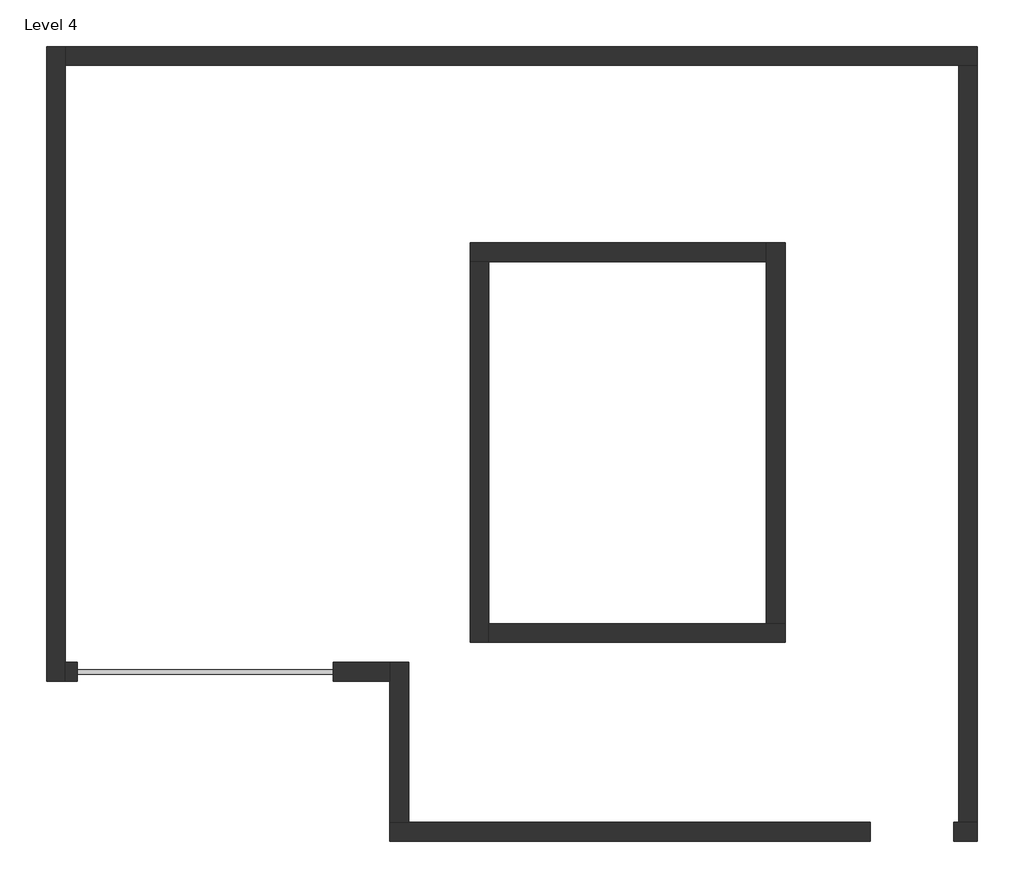
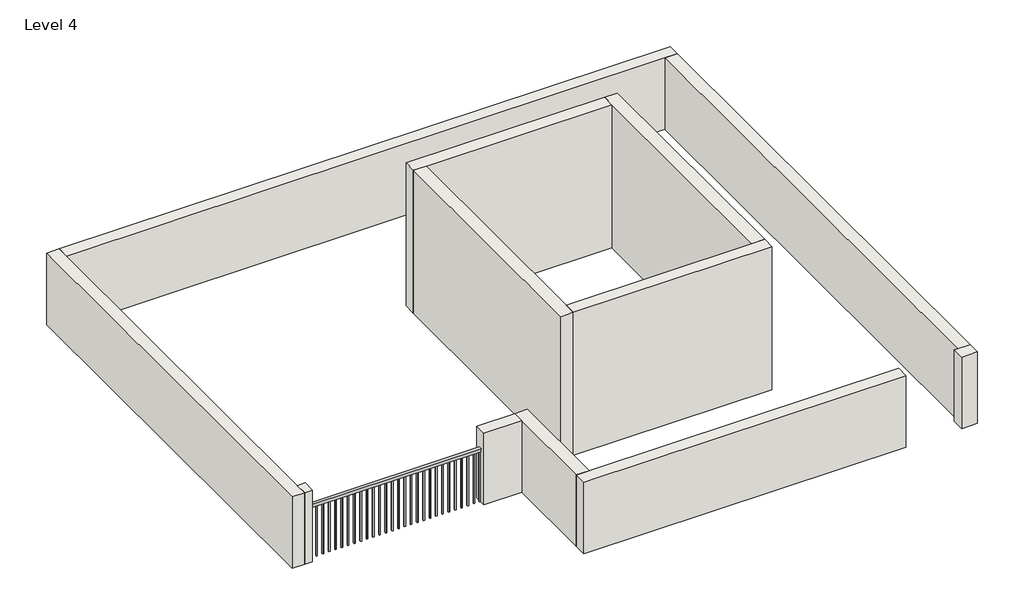
# One storey: 10 walls, 1 railing.
"""IFC4 building model written with IfcOpenShell, lengths in millimetres."""

from ifc_helpers import new_model, si_unit, frame, origin, place, context, project, spatial, polyline, outline, extrude, faceted_brep, element, save

model = new_model("IFC4")

# Units and contexts
model_context = context("Model", 3, world=origin())
ifc_project = project(units=[si_unit("LENGTHUNIT", "METRE", prefix="MILLI")], contexts=[model_context])

# Site, building, storey
site = spatial("IfcSite", under=ifc_project)
building = spatial("IfcBuilding", under=site)
storey = spatial("IfcBuildingStorey", under=building, Name="Level 4", Elevation=3810.0)

# Railing
placement = place(None, origin())
element("IfcRailing", 1, ObjectType="Handrail - Rectangular", at=placement, inside=storey, context=model_context, shape_type="SweptSolid", body=[
    extrude(outline(polyline([(-5551.2524032, 7396.0433441), (-5551.2524032, 7345.2433441), (-8317.8992801, 7345.2433441), (-8317.8992801, 7396.0433441), (-5551.2524032, 7396.0433441)])), frame((0.0, 0.0, 4673.6), z_axis=(0.0, 0.0, 1.0), x_axis=(1.0, 0.0, 0.0)), (0.0, 0.0, 1.0), 50.8),
    extrude(outline(polyline([(-8284.9274032, 7380.1683441), (-8284.9274032, 7361.1183441), (-8303.9774032, 7361.1183441), (-8303.9774032, 7380.1683441), (-8284.9274032, 7380.1683441)])), frame((0.0, 0.0, 3810.0), z_axis=(0.0, 0.0, 1.0), x_axis=(1.0, 0.0, 0.0)), (0.0, 0.0, 1.0), 863.6),
    extrude(outline(polyline([(-8183.3274032, 7380.1683441), (-8183.3274032, 7361.1183441), (-8202.3774032, 7361.1183441), (-8202.3774032, 7380.1683441), (-8183.3274032, 7380.1683441)])), frame((0.0, 0.0, 3810.0), z_axis=(0.0, 0.0, 1.0), x_axis=(1.0, 0.0, 0.0)), (0.0, 0.0, 1.0), 863.6),
    extrude(outline(polyline([(-8081.7274032, 7380.1683441), (-8081.7274032, 7361.1183441), (-8100.7774032, 7361.1183441), (-8100.7774032, 7380.1683441), (-8081.7274032, 7380.1683441)])), frame((0.0, 0.0, 3810.0), z_axis=(0.0, 0.0, 1.0), x_axis=(1.0, 0.0, 0.0)), (0.0, 0.0, 1.0), 863.6),
    extrude(outline(polyline([(-7980.1274032, 7380.1683441), (-7980.1274032, 7361.1183441), (-7999.1774032, 7361.1183441), (-7999.1774032, 7380.1683441), (-7980.1274032, 7380.1683441)])), frame((0.0, 0.0, 3810.0), z_axis=(0.0, 0.0, 1.0), x_axis=(1.0, 0.0, 0.0)), (0.0, 0.0, 1.0), 863.6),
    extrude(outline(polyline([(-7878.5274032, 7380.1683441), (-7878.5274032, 7361.1183441), (-7897.5774032, 7361.1183441), (-7897.5774032, 7380.1683441), (-7878.5274032, 7380.1683441)])), frame((0.0, 0.0, 3810.0), z_axis=(0.0, 0.0, 1.0), x_axis=(1.0, 0.0, 0.0)), (0.0, 0.0, 1.0), 863.6),
    extrude(outline(polyline([(-7776.9274032, 7380.1683441), (-7776.9274032, 7361.1183441), (-7795.9774032, 7361.1183441), (-7795.9774032, 7380.1683441), (-7776.9274032, 7380.1683441)])), frame((0.0, 0.0, 3810.0), z_axis=(0.0, 0.0, 1.0), x_axis=(1.0, 0.0, 0.0)), (0.0, 0.0, 1.0), 863.6),
    extrude(outline(polyline([(-7675.3274032, 7380.1683441), (-7675.3274032, 7361.1183441), (-7694.3774032, 7361.1183441), (-7694.3774032, 7380.1683441), (-7675.3274032, 7380.1683441)])), frame((0.0, 0.0, 3810.0), z_axis=(0.0, 0.0, 1.0), x_axis=(1.0, 0.0, 0.0)), (0.0, 0.0, 1.0), 863.6),
    extrude(outline(polyline([(-7573.7274032, 7380.1683441), (-7573.7274032, 7361.1183441), (-7592.7774032, 7361.1183441), (-7592.7774032, 7380.1683441), (-7573.7274032, 7380.1683441)])), frame((0.0, 0.0, 3810.0), z_axis=(0.0, 0.0, 1.0), x_axis=(1.0, 0.0, 0.0)), (0.0, 0.0, 1.0), 863.6),
    extrude(outline(polyline([(-7472.1274032, 7380.1683441), (-7472.1274032, 7361.1183441), (-7491.1774032, 7361.1183441), (-7491.1774032, 7380.1683441), (-7472.1274032, 7380.1683441)])), frame((0.0, 0.0, 3810.0), z_axis=(0.0, 0.0, 1.0), x_axis=(1.0, 0.0, 0.0)), (0.0, 0.0, 1.0), 863.6),
    extrude(outline(polyline([(-7370.5274032, 7380.1683441), (-7370.5274032, 7361.1183441), (-7389.5774032, 7361.1183441), (-7389.5774032, 7380.1683441), (-7370.5274032, 7380.1683441)])), frame((0.0, 0.0, 3810.0), z_axis=(0.0, 0.0, 1.0), x_axis=(1.0, 0.0, 0.0)), (0.0, 0.0, 1.0), 863.6),
    extrude(outline(polyline([(-7268.9274032, 7380.1683441), (-7268.9274032, 7361.1183441), (-7287.9774032, 7361.1183441), (-7287.9774032, 7380.1683441), (-7268.9274032, 7380.1683441)])), frame((0.0, 0.0, 3810.0), z_axis=(0.0, 0.0, 1.0), x_axis=(1.0, 0.0, 0.0)), (0.0, 0.0, 1.0), 863.6),
    extrude(outline(polyline([(-7167.3274032, 7380.1683441), (-7167.3274032, 7361.1183441), (-7186.3774032, 7361.1183441), (-7186.3774032, 7380.1683441), (-7167.3274032, 7380.1683441)])), frame((0.0, 0.0, 3810.0), z_axis=(0.0, 0.0, 1.0), x_axis=(1.0, 0.0, 0.0)), (0.0, 0.0, 1.0), 863.6),
    extrude(outline(polyline([(-7065.7274032, 7380.1683441), (-7065.7274032, 7361.1183441), (-7084.7774032, 7361.1183441), (-7084.7774032, 7380.1683441), (-7065.7274032, 7380.1683441)])), frame((0.0, 0.0, 3810.0), z_axis=(0.0, 0.0, 1.0), x_axis=(1.0, 0.0, 0.0)), (0.0, 0.0, 1.0), 863.6),
    extrude(outline(polyline([(-6964.1274032, 7380.1683441), (-6964.1274032, 7361.1183441), (-6983.1774032, 7361.1183441), (-6983.1774032, 7380.1683441), (-6964.1274032, 7380.1683441)])), frame((0.0, 0.0, 3810.0), z_axis=(0.0, 0.0, 1.0), x_axis=(1.0, 0.0, 0.0)), (0.0, 0.0, 1.0), 863.6),
    extrude(outline(polyline([(-6862.5274032, 7380.1683441), (-6862.5274032, 7361.1183441), (-6881.5774032, 7361.1183441), (-6881.5774032, 7380.1683441), (-6862.5274032, 7380.1683441)])), frame((0.0, 0.0, 3810.0), z_axis=(0.0, 0.0, 1.0), x_axis=(1.0, 0.0, 0.0)), (0.0, 0.0, 1.0), 863.6),
    extrude(outline(polyline([(-6760.9274032, 7380.1683441), (-6760.9274032, 7361.1183441), (-6779.9774032, 7361.1183441), (-6779.9774032, 7380.1683441), (-6760.9274032, 7380.1683441)])), frame((0.0, 0.0, 3810.0), z_axis=(0.0, 0.0, 1.0), x_axis=(1.0, 0.0, 0.0)), (0.0, 0.0, 1.0), 863.6),
    extrude(outline(polyline([(-6659.3274032, 7380.1683441), (-6659.3274032, 7361.1183441), (-6678.3774032, 7361.1183441), (-6678.3774032, 7380.1683441), (-6659.3274032, 7380.1683441)])), frame((0.0, 0.0, 3810.0), z_axis=(0.0, 0.0, 1.0), x_axis=(1.0, 0.0, 0.0)), (0.0, 0.0, 1.0), 863.6),
    extrude(outline(polyline([(-6557.7274032, 7380.1683441), (-6557.7274032, 7361.1183441), (-6576.7774032, 7361.1183441), (-6576.7774032, 7380.1683441), (-6557.7274032, 7380.1683441)])), frame((0.0, 0.0, 3810.0), z_axis=(0.0, 0.0, 1.0), x_axis=(1.0, 0.0, 0.0)), (0.0, 0.0, 1.0), 863.6),
    extrude(outline(polyline([(-6456.1274032, 7380.1683441), (-6456.1274032, 7361.1183441), (-6475.1774032, 7361.1183441), (-6475.1774032, 7380.1683441), (-6456.1274032, 7380.1683441)])), frame((0.0, 0.0, 3810.0), z_axis=(0.0, 0.0, 1.0), x_axis=(1.0, 0.0, 0.0)), (0.0, 0.0, 1.0), 863.6),
    extrude(outline(polyline([(-6354.5274032, 7380.1683441), (-6354.5274032, 7361.1183441), (-6373.5774032, 7361.1183441), (-6373.5774032, 7380.1683441), (-6354.5274032, 7380.1683441)])), frame((0.0, 0.0, 3810.0), z_axis=(0.0, 0.0, 1.0), x_axis=(1.0, 0.0, 0.0)), (0.0, 0.0, 1.0), 863.6),
    extrude(outline(polyline([(-6252.9274032, 7380.1683441), (-6252.9274032, 7361.1183441), (-6271.9774032, 7361.1183441), (-6271.9774032, 7380.1683441), (-6252.9274032, 7380.1683441)])), frame((0.0, 0.0, 3810.0), z_axis=(0.0, 0.0, 1.0), x_axis=(1.0, 0.0, 0.0)), (0.0, 0.0, 1.0), 863.6),
    extrude(outline(polyline([(-6151.3274032, 7380.1683441), (-6151.3274032, 7361.1183441), (-6170.3774032, 7361.1183441), (-6170.3774032, 7380.1683441), (-6151.3274032, 7380.1683441)])), frame((0.0, 0.0, 3810.0), z_axis=(0.0, 0.0, 1.0), x_axis=(1.0, 0.0, 0.0)), (0.0, 0.0, 1.0), 863.6),
    extrude(outline(polyline([(-6049.7274032, 7380.1683441), (-6049.7274032, 7361.1183441), (-6068.7774032, 7361.1183441), (-6068.7774032, 7380.1683441), (-6049.7274032, 7380.1683441)])), frame((0.0, 0.0, 3810.0), z_axis=(0.0, 0.0, 1.0), x_axis=(1.0, 0.0, 0.0)), (0.0, 0.0, 1.0), 863.6),
    extrude(outline(polyline([(-5948.1274032, 7380.1683441), (-5948.1274032, 7361.1183441), (-5967.1774032, 7361.1183441), (-5967.1774032, 7380.1683441), (-5948.1274032, 7380.1683441)])), frame((0.0, 0.0, 3810.0), z_axis=(0.0, 0.0, 1.0), x_axis=(1.0, 0.0, 0.0)), (0.0, 0.0, 1.0), 863.6),
    extrude(outline(polyline([(-5846.5274032, 7380.1683441), (-5846.5274032, 7361.1183441), (-5865.5774032, 7361.1183441), (-5865.5774032, 7380.1683441), (-5846.5274032, 7380.1683441)])), frame((0.0, 0.0, 3810.0), z_axis=(0.0, 0.0, 1.0), x_axis=(1.0, 0.0, 0.0)), (0.0, 0.0, 1.0), 863.6),
    extrude(outline(polyline([(-5744.9274032, 7380.1683441), (-5744.9274032, 7361.1183441), (-5763.9774032, 7361.1183441), (-5763.9774032, 7380.1683441), (-5744.9274032, 7380.1683441)])), frame((0.0, 0.0, 3810.0), z_axis=(0.0, 0.0, 1.0), x_axis=(1.0, 0.0, 0.0)), (0.0, 0.0, 1.0), 863.6),
    extrude(outline(polyline([(-5643.3274032, 7380.1683441), (-5643.3274032, 7361.1183441), (-5662.3774032, 7361.1183441), (-5662.3774032, 7380.1683441), (-5643.3274032, 7380.1683441)])), frame((0.0, 0.0, 3810.0), z_axis=(0.0, 0.0, 1.0), x_axis=(1.0, 0.0, 0.0)), (0.0, 0.0, 1.0), 863.6),
    extrude(outline(polyline([(-8298.8492801, 7380.1683441), (-8298.8492801, 7361.1183441), (-8317.8992801, 7361.1183441), (-8317.8992801, 7380.1683441), (-8298.8492801, 7380.1683441)])), frame((0.0, 0.0, 3810.0), z_axis=(0.0, 0.0, 1.0), x_axis=(1.0, 0.0, 0.0)), (0.0, 0.0, 1.0), 863.6),
    extrude(outline(polyline([(-5551.2524032, 7380.1683441), (-5551.2524032, 7361.1183441), (-5570.3024032, 7361.1183441), (-5570.3024032, 7380.1683441), (-5551.2524032, 7380.1683441)])), frame((0.0, 0.0, 3810.0), z_axis=(0.0, 0.0, 1.0), x_axis=(1.0, 0.0, 0.0)), (0.0, 0.0, 1.0), 863.6),
])

# Walls
element("IfcWall", 2, ObjectType="9\" wall", at=placement, inside=storey, context=model_context, shape_type="Brep", body=[
    faceted_brep([(-8443.959401, 7269.0433441, 3810.0), (-8443.959401, 7472.2433441, 3810.0), (-8443.959401, 13923.8433441, 3810.0), (-8443.959401, 14127.0433441, 3810.0), (-8443.959401, 14127.0433441, 5029.2), (-8443.959401, 13923.8433441, 5029.2), (-8443.959401, 7472.2433441, 5029.2), (-8443.959401, 7269.0433441, 5029.2), (-8647.159401, 7269.0433441, 3810.0), (-8647.159401, 7269.0433441, 5029.2), (-8647.159401, 14127.0433441, 5029.2), (-8647.159401, 14127.0433441, 3810.0)], [[[0, 1, 2, 3, 4, 5, 6, 7]], [[8, 9, 10, 11]], [[3, 2, 1, 0, 8, 11]], [[7, 6, 5, 4, 10, 9]], [[4, 3, 11, 10]], [[0, 7, 9, 8]]]),
])
element("IfcWall", 3, ObjectType="9\" wall", at=placement, inside=storey, context=model_context, shape_type="Brep", body=[
    faceted_brep([(-8443.959401, 13923.8433441, 3810.0), (1208.040599, 13923.8433441, 3810.0), (1411.240599, 13923.8433441, 3810.0), (1411.240599, 13923.8433441, 5029.2), (1208.040599, 13923.8433441, 5029.2), (-8443.959401, 13923.8433441, 5029.2), (-8443.959401, 14127.0433441, 3810.0), (-8443.959401, 14127.0433441, 5029.2), (1411.240599, 14127.0433441, 5029.2), (1411.240599, 14127.0433441, 3810.0)], [[[0, 1, 2, 3, 4, 5]], [[6, 7, 8, 9]], [[2, 1, 0, 6, 9]], [[5, 4, 3, 8, 7]], [[0, 5, 7, 6]], [[3, 2, 9, 8]]]),
])
element("IfcWall", 4, ObjectType="9\" wall", at=placement, inside=storey, context=model_context, shape_type="SweptSolid", body=[
    extrude(outline(polyline([(1208.040599, 5745.0433441), (1208.040599, 13923.8433441), (1411.240599, 13923.8433441), (1411.240599, 5745.0433441), (1208.040599, 5745.0433441)])), frame((0.0, 0.0, 3810.0), z_axis=(0.0, 0.0, 1.0), x_axis=(1.0, 0.0, 0.0)), (0.0, 0.0, 1.0), 1219.2),
])
element("IfcWall", 5, ObjectType="9\" wall", at=placement, inside=storey, context=model_context, shape_type="Brep", body=[
    faceted_brep([(-4938.759401, 5745.0433441, 3810.0), (-4938.759401, 5745.0433441, 5029.2), (-4735.559401, 5745.0433441, 5029.2), (255.1235865, 5745.0433441, 5029.2), (255.1235865, 5745.0433441, 3810.0), (-4735.559401, 5745.0433441, 3810.0), (-4938.759401, 5541.8433441, 5029.2), (-4938.759401, 5541.8433441, 3810.0), (255.1235865, 5541.8433441, 3810.0), (255.1235865, 5541.8433441, 5029.2)], [[[0, 1, 2, 3, 4, 5]], [[6, 7, 8, 9]], [[7, 0, 5, 4, 8]], [[1, 6, 9, 3, 2]], [[1, 0, 7, 6]], [[4, 3, 9, 8]]]),
    faceted_brep([(1411.240599, 5745.0433441, 5029.2), (1411.240599, 5745.0433441, 3810.0), (1208.040599, 5745.0433441, 3810.0), (1157.240599, 5745.0433441, 3810.0), (1157.240599, 5745.0433441, 5029.2), (1208.040599, 5745.0433441, 5029.2), (1411.240599, 5541.8433441, 3810.0), (1411.240599, 5541.8433441, 5029.2), (1157.240599, 5541.8433441, 5029.2), (1157.240599, 5541.8433441, 3810.0)], [[[0, 1, 2, 3, 4, 5]], [[6, 7, 8, 9]], [[1, 6, 9, 3, 2]], [[7, 0, 5, 4, 8]], [[4, 3, 9, 8]], [[1, 0, 7, 6]]]),
])
element("IfcWall", 6, ObjectType="9\" wall", at=placement, inside=storey, context=model_context, shape_type="Brep", body=[
    faceted_brep([(-4735.559401, 5745.0433441, 3810.0), (-4735.559401, 7472.2433441, 3810.0), (-4735.559401, 7472.2433441, 5029.2), (-4735.559401, 5745.0433441, 5029.2), (-4938.759401, 5745.0433441, 3810.0), (-4938.759401, 5745.0433441, 5029.2), (-4938.759401, 7269.0433441, 5029.2), (-4938.759401, 7472.2433441, 5029.2), (-4938.759401, 7472.2433441, 3810.0), (-4938.759401, 7269.0433441, 3810.0)], [[[0, 1, 2, 3]], [[4, 5, 6, 7, 8, 9]], [[1, 0, 4, 9, 8]], [[3, 2, 7, 6, 5]], [[0, 3, 5, 4]], [[2, 1, 8, 7]]]),
])
element("IfcWall", 7, ObjectType="9\" wall", at=placement, inside=storey, context=model_context, shape_type="SweptSolid", body=[
    extrude(outline(polyline([(-8443.959401, 7269.0433441), (-8443.959401, 7472.2433441), (-8317.8992801, 7472.2433441), (-8317.8992801, 7269.0433441), (-8443.959401, 7269.0433441)])), frame((0.0, 0.0, 3810.0), z_axis=(0.0, 0.0, 1.0), x_axis=(1.0, 0.0, 0.0)), (0.0, 0.0, 1.0), 1219.2),
    extrude(outline(polyline([(-4938.759401, 7472.2433441), (-4938.759401, 7269.0433441), (-5551.2524032, 7269.0433441), (-5551.2524032, 7472.2433441), (-4938.759401, 7472.2433441)])), frame((0.0, 0.0, 3810.0), z_axis=(0.0, 0.0, 1.0), x_axis=(1.0, 0.0, 0.0)), (0.0, 0.0, 1.0), 1219.2),
])
element("IfcWall", 8, ObjectType="9\" wall", at=placement, inside=storey, context=model_context, shape_type="Brep", body=[
    faceted_brep([(-4070.3116656, 11803.4455153, 3810.0), (-3867.1116656, 11803.4455153, 3810.0), (-869.9116656, 11803.4455153, 3810.0), (-869.9116656, 11803.4455153, 6248.4), (-3867.1116656, 11803.4455153, 6248.4), (-4070.3116656, 11803.4455153, 6248.4), (-4070.3116656, 12006.6455153, 3810.0), (-4070.3116656, 12006.6455153, 6248.4), (-869.9116656, 12006.6455153, 6248.4), (-869.9116656, 12006.6455153, 3810.0)], [[[0, 1, 2, 3, 4, 5]], [[6, 7, 8, 9]], [[2, 1, 0, 6, 9]], [[5, 4, 3, 8, 7]], [[0, 5, 7, 6]], [[3, 2, 9, 8]]]),
])
element("IfcWall", 9, ObjectType="9\" wall", at=placement, inside=storey, context=model_context, shape_type="Brep", body=[
    faceted_brep([(-3867.1116656, 7688.6455153, 3810.0), (-3867.1116656, 7891.8455153, 3810.0), (-3867.1116656, 11803.4455153, 3810.0), (-3867.1116656, 11803.4455153, 6248.4), (-3867.1116656, 7891.8455153, 6248.4), (-3867.1116656, 7688.6455153, 6248.4), (-4070.3116656, 7688.6455153, 3810.0), (-4070.3116656, 7688.6455153, 6248.4), (-4070.3116656, 11803.4455153, 6248.4), (-4070.3116656, 11803.4455153, 3810.0)], [[[0, 1, 2, 3, 4, 5]], [[6, 7, 8, 9]], [[2, 1, 0, 6, 9]], [[5, 4, 3, 8, 7]], [[0, 5, 7, 6]], [[3, 2, 9, 8]]]),
])
element("IfcWall", 10, ObjectType="9\" wall", at=placement, inside=storey, context=model_context, shape_type="Brep", body=[
    faceted_brep([(-666.7116656, 7891.8455153, 3810.0), (-869.9116656, 7891.8455153, 3810.0), (-3867.1116656, 7891.8455153, 3810.0), (-3867.1116656, 7891.8455153, 6248.4), (-869.9116656, 7891.8455153, 6248.4), (-666.7116656, 7891.8455153, 6248.4), (-666.7116656, 7688.6455153, 3810.0), (-666.7116656, 7688.6455153, 6248.4), (-3867.1116656, 7688.6455153, 6248.4), (-3867.1116656, 7688.6455153, 3810.0)], [[[0, 1, 2, 3, 4, 5]], [[6, 7, 8, 9]], [[2, 1, 0, 6, 9]], [[5, 4, 3, 8, 7]], [[0, 5, 7, 6]], [[3, 2, 9, 8]]]),
])
element("IfcWall", 11, ObjectType="9\" wall", at=placement, inside=storey, context=model_context, shape_type="Brep", body=[
    faceted_brep([(-869.9116656, 12006.6455153, 3810.0), (-869.9116656, 11803.4455153, 3810.0), (-869.9116656, 7891.8455153, 3810.0), (-869.9116656, 7891.8455153, 6248.4), (-869.9116656, 11803.4455153, 6248.4), (-869.9116656, 12006.6455153, 6248.4), (-666.7116656, 12006.6455153, 3810.0), (-666.7116656, 12006.6455153, 6248.4), (-666.7116656, 7891.8455153, 6248.4), (-666.7116656, 7891.8455153, 3810.0)], [[[0, 1, 2, 3, 4, 5]], [[6, 7, 8, 9]], [[2, 1, 0, 6, 9]], [[5, 4, 3, 8, 7]], [[0, 5, 7, 6]], [[3, 2, 9, 8]]]),
])

save(model, "model.ifc")

# Revit data of these elements
# Type "Handrail - Rectangular"
#   Assembly Code = "C2010400"
#   built-in parameter 1008612 = 0.0416667 (stored number, unit not read)
#   built-in parameter 1008611 = 0.0416667 (stored number, unit not read)
#   built-in parameter 1008609 = 0.333333 (stored number, unit not read)
#   built-in parameter 1008604 = 0.166667 (stored number, unit not read)
#   built-in parameter 1008603 = 0.166667 (stored number, unit not read)
#   Railing Height = 3' - 0"
#   built-in parameter 1008630 = 2
#   built-in parameter 1008610 = 2
#   built-in parameter 1008618 = Baluster - Square : 3/4"
# Type "9\" wall"
#   Assembly Code = "B2010"
#   Layers, outside or top first: 0' - 8" no material (function 1)
# Element 1 (IfcRailing, "Handrail - Rectangular")
#   Phase Created = New Construction
# Elements 2, 3, 4, 5, 6, 7 (IfcWall, "9\" wall")
#   Top Offset = 0' - 0"
#   Base Offset = 0' - 0"
#   wall height = 4' - 0"
#   Phase Created = New Construction
#   Base Constraint = Level 4
#   Top Constraint = Level 5
#   Materials on its faces: "Default Wall"
# Elements 8, 9, 10, 11 (IfcWall, "9\" wall")
#   Top Offset = 0' - 0"
#   Base Offset = 0' - 0"
#   Unconnected Height = 8' - 0"
#   wall height = 8' - 0"
#   Phase Created = New Construction
#   Base Constraint = Level 4
#   Materials on its faces: "Default Wall"
# Materials
#   "Default Wall": colour RGB 128 128 128, transparency 0, Cost = 0
